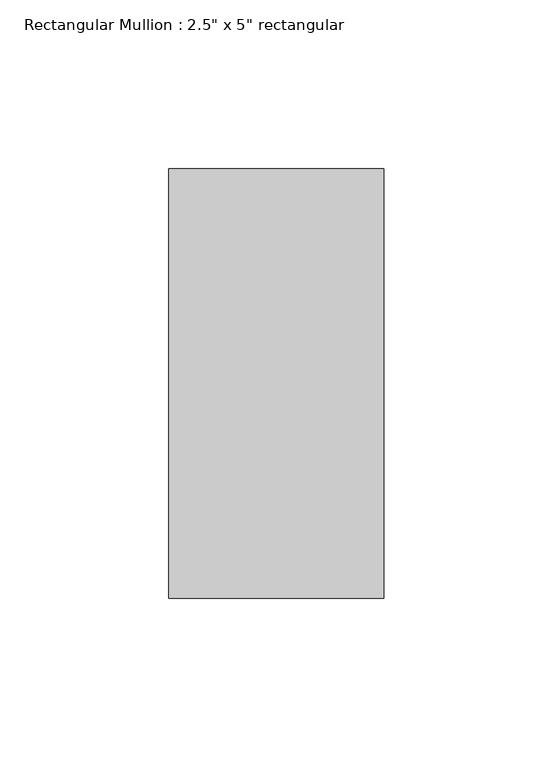
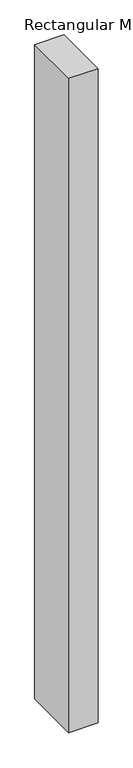
"""IFC4 building model written with IfcOpenShell, lengths in millimetres: member geometry."""

from ifc_helpers import new_model, si_unit, frame, origin, place, context, project, spatial, polyline, outline, extrude, source, transform, mapped, element, save


def member_143ec642(model_context):
    return source(origin(), model_context, "Body", "SweptSolid", [
        extrude(outline(polyline([(0.0, 63.5), (0.0, -63.5), (-63.5, -63.5), (-63.5, 63.5), (0.0, 63.5)])), frame((0.0, 0.0, -1498.695751), z_axis=(0.0, 0.0, 1.0), x_axis=(1.0, 0.0, 0.0)), (0.0, 0.0, 1.0), 1498.695751),
    ])


if __name__ == "__main__":
    model = new_model("IFC4")
    model_context = context("Model", 3, world=origin())
    ifc_project = project(units=[si_unit("LENGTHUNIT", "METRE", prefix="MILLI")], contexts=[model_context])
    site = spatial("IfcSite", under=ifc_project)
    building = spatial("IfcBuilding", under=site)
    placement = place(None, origin())
    member_shape = member_143ec642(model_context)
    element("IfcMember", 1, ObjectType="Rectangular Mullion : 2.5\" x 5\" rectangular", at=placement, inside=building, context=model_context, shape_type="MappedRepresentation", body=[
        mapped(member_shape, transform((0.0, 0.0, 0.0), x_axis=(1.0, 0.0, 0.0), y_axis=(0.0, 1.0, 0.0), z_axis=(0.0, 0.0, 1.0))),
    ])
    save(model, "model.ifc")

# Revit data of these elements
# Type "Rectangular Mullion : 2.5\" x 5\" rectangular"
#   built-in parameter 1007304 = 0.416667 (stored number, unit not read)
#   built-in parameter 1007301 = 0.104167 (stored number, unit not read)
#   built-in parameter 1007300 = 0.104167 (stored number, unit not read)
# Element 1 (IfcMember, "Rectangular Mullion : 2.5\" x 5\" rectangular")
#   Materials on its faces: "Aluminum"
# Materials
#   "Aluminum": class "Metal", colour RGB 247 247 247, transparency 0, Description = "Aluminum 6061", Cost = 0
